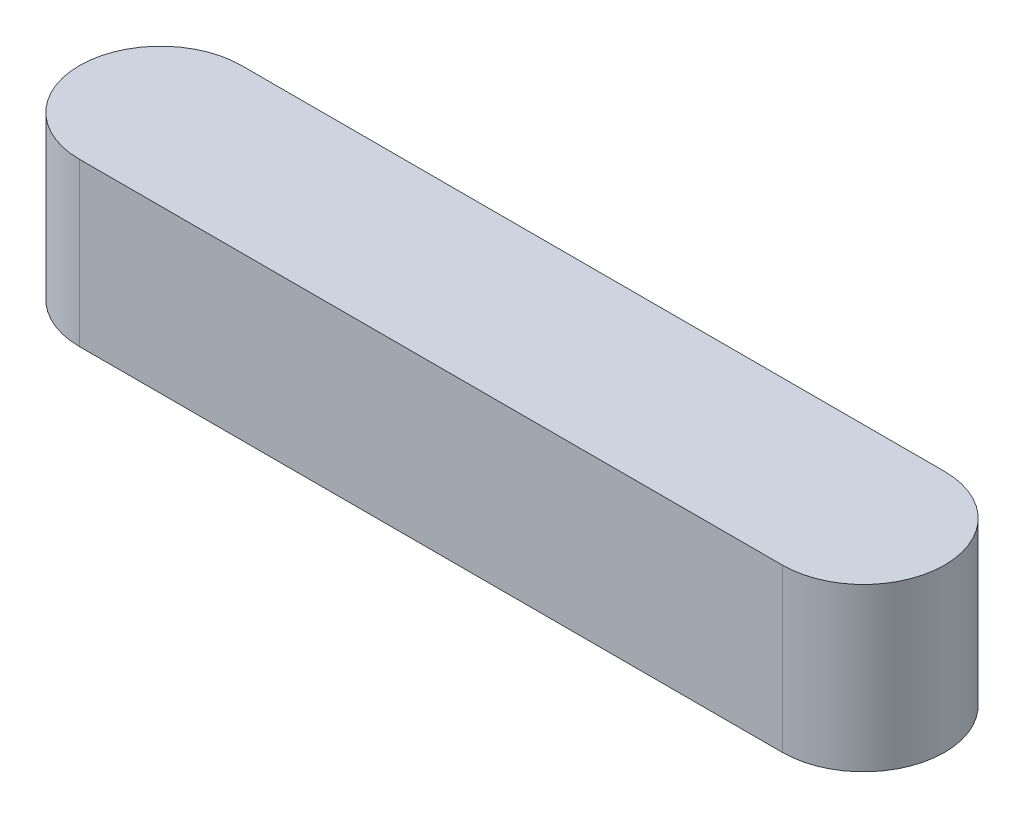
ISO-10303-21;
HEADER;
FILE_DESCRIPTION(('STEP AP214'),'2;1');
FILE_NAME('part.step','',(''),(''),'','','');
FILE_SCHEMA(('AUTOMOTIVE_DESIGN { 1 0 10303 214 1 1 1 1 }'));
ENDSEC;
DATA;
#1=APPLICATION_CONTEXT('core data for automotive mechanical design processes');
#2=APPLICATION_PROTOCOL_DEFINITION('international standard','automotive_design',2000,#1);
#3=PRODUCT_CONTEXT('',#1,'mechanical');
#4=PRODUCT('Part','Part','',(#3));
#5=PRODUCT_RELATED_PRODUCT_CATEGORY('part','',(#4));
#6=PRODUCT_DEFINITION_FORMATION('','',#4);
#7=PRODUCT_DEFINITION_CONTEXT('part definition',#1,'design');
#8=PRODUCT_DEFINITION('design','',#6,#7);
#9=PRODUCT_DEFINITION_SHAPE('','',#8);
#10=(LENGTH_UNIT() NAMED_UNIT(*) SI_UNIT(.MILLI.,.METRE.));
#11=(NAMED_UNIT(*) PLANE_ANGLE_UNIT() SI_UNIT($,.RADIAN.));
#12=(NAMED_UNIT(*) SI_UNIT($,.STERADIAN.) SOLID_ANGLE_UNIT());
#13=UNCERTAINTY_MEASURE_WITH_UNIT(LENGTH_MEASURE(1.E-05),#10,'distance_accuracy_value','');
#14=(GEOMETRIC_REPRESENTATION_CONTEXT(3) GLOBAL_UNCERTAINTY_ASSIGNED_CONTEXT((#13)) GLOBAL_UNIT_ASSIGNED_CONTEXT((#10,
#11,#12)) REPRESENTATION_CONTEXT('',''));
#15=CARTESIAN_POINT('',(0.,0.,0.));
#16=DIRECTION('',(0.,0.,1.));
#17=DIRECTION('',(1.,0.,0.));
#18=AXIS2_PLACEMENT_3D('',#15,#16,#17);
#19=CARTESIAN_POINT('',(-13.,6.,0.));
#20=DIRECTION('',(0.,-1.,0.));
#21=DIRECTION('',(0.,0.,-1.));
#22=AXIS2_PLACEMENT_3D('',#19,#20,#21);
#23=CYLINDRICAL_SURFACE('',#22,3.);
#24=CARTESIAN_POINT('',(-13.,0.,0.));
#25=DIRECTION('',(0.,1.,0.));
#26=DIRECTION('',(0.,0.,1.));
#27=AXIS2_PLACEMENT_3D('',#24,#25,#26);
#28=CIRCLE('',#27,3.);
#29=CARTESIAN_POINT('',(-13.,0.,-3.));
#30=VERTEX_POINT('',#29);
#31=CARTESIAN_POINT('',(-13.,0.,3.));
#32=VERTEX_POINT('',#31);
#33=EDGE_CURVE('E105',#30,#32,#28,.T.);
#34=ORIENTED_EDGE('',*,*,#33,.T.);
#35=DIRECTION('',(0.,-1.,0.));
#36=VECTOR('',#35,1.);
#37=CARTESIAN_POINT('',(-13.,6.,3.));
#38=LINE('',#37,#36);
#39=CARTESIAN_POINT('',(-13.,6.,3.));
#40=VERTEX_POINT('',#39);
#41=EDGE_CURVE('E11',#40,#32,#38,.T.);
#42=ORIENTED_EDGE('',*,*,#41,.F.);
#43=CARTESIAN_POINT('',(-13.,6.,0.));
#44=DIRECTION('',(0.,1.,0.));
#45=DIRECTION('',(0.,0.,1.));
#46=AXIS2_PLACEMENT_3D('',#43,#44,#45);
#47=CIRCLE('',#46,3.);
#48=CARTESIAN_POINT('',(-13.,6.,-3.));
#49=VERTEX_POINT('',#48);
#50=EDGE_CURVE('E89',#49,#40,#47,.T.);
#51=ORIENTED_EDGE('',*,*,#50,.F.);
#52=DIRECTION('',(0.,-1.,0.));
#53=VECTOR('',#52,1.);
#54=CARTESIAN_POINT('',(-13.,6.,-3.));
#55=LINE('',#54,#53);
#56=EDGE_CURVE('E98',#49,#30,#55,.T.);
#57=ORIENTED_EDGE('',*,*,#56,.T.);
#58=EDGE_LOOP('',(#34,#42,#51,#57));
#59=FACE_BOUND('',#58,.T.);
#60=ADVANCED_FACE('F39',(#59),#23,.T.);
#61=CARTESIAN_POINT('',(-13.,6.,3.));
#62=DIRECTION('',(0.,0.,-1.));
#63=DIRECTION('',(-1.,0.,0.));
#64=AXIS2_PLACEMENT_3D('',#61,#62,#63);
#65=PLANE('',#64);
#66=DIRECTION('',(1.,0.,0.));
#67=VECTOR('',#66,1.);
#68=CARTESIAN_POINT('',(-13.,0.,3.));
#69=LINE('',#68,#67);
#70=CARTESIAN_POINT('',(13.,0.,3.));
#71=VERTEX_POINT('',#70);
#72=EDGE_CURVE('E94',#32,#71,#69,.T.);
#73=ORIENTED_EDGE('',*,*,#72,.T.);
#74=DIRECTION('',(0.,-1.,0.));
#75=VECTOR('',#74,1.);
#76=CARTESIAN_POINT('',(13.,6.,3.));
#77=LINE('',#76,#75);
#78=CARTESIAN_POINT('',(13.,6.,3.));
#79=VERTEX_POINT('',#78);
#80=EDGE_CURVE('E50',#79,#71,#77,.T.);
#81=ORIENTED_EDGE('',*,*,#80,.F.);
#82=DIRECTION('',(1.,0.,0.));
#83=VECTOR('',#82,1.);
#84=CARTESIAN_POINT('',(-13.,6.,3.));
#85=LINE('',#84,#83);
#86=EDGE_CURVE('E85',#40,#79,#85,.T.);
#87=ORIENTED_EDGE('',*,*,#86,.F.);
#88=ORIENTED_EDGE('',*,*,#41,.T.);
#89=EDGE_LOOP('',(#73,#81,#87,#88));
#90=FACE_BOUND('',#89,.T.);
#91=ADVANCED_FACE('F91',(#90),#65,.F.);
#92=CARTESIAN_POINT('',(13.,6.,0.));
#93=DIRECTION('',(0.,-1.,0.));
#94=DIRECTION('',(0.,0.,-1.));
#95=AXIS2_PLACEMENT_3D('',#92,#93,#94);
#96=CYLINDRICAL_SURFACE('',#95,3.);
#97=CARTESIAN_POINT('',(13.,0.,0.));
#98=DIRECTION('',(0.,1.,0.));
#99=DIRECTION('',(0.,0.,1.));
#100=AXIS2_PLACEMENT_3D('',#97,#98,#99);
#101=CIRCLE('',#100,3.);
#102=CARTESIAN_POINT('',(13.,0.,-3.));
#103=VERTEX_POINT('',#102);
#104=EDGE_CURVE('E75',#71,#103,#101,.T.);
#105=ORIENTED_EDGE('',*,*,#104,.T.);
#106=DIRECTION('',(0.,-1.,0.));
#107=VECTOR('',#106,1.);
#108=CARTESIAN_POINT('',(13.,6.,-3.));
#109=LINE('',#108,#107);
#110=CARTESIAN_POINT('',(13.,6.,-3.));
#111=VERTEX_POINT('',#110);
#112=EDGE_CURVE('E92',#111,#103,#109,.T.);
#113=ORIENTED_EDGE('',*,*,#112,.F.);
#114=CARTESIAN_POINT('',(13.,6.,0.));
#115=DIRECTION('',(0.,1.,0.));
#116=DIRECTION('',(0.,0.,1.));
#117=AXIS2_PLACEMENT_3D('',#114,#115,#116);
#118=CIRCLE('',#117,3.);
#119=EDGE_CURVE('E86',#79,#111,#118,.T.);
#120=ORIENTED_EDGE('',*,*,#119,.F.);
#121=ORIENTED_EDGE('',*,*,#80,.T.);
#122=EDGE_LOOP('',(#105,#113,#120,#121));
#123=FACE_BOUND('',#122,.T.);
#124=ADVANCED_FACE('F96',(#123),#96,.T.);
#125=CARTESIAN_POINT('',(-13.,6.,-3.));
#126=DIRECTION('',(0.,0.,1.));
#127=DIRECTION('',(1.,0.,0.));
#128=AXIS2_PLACEMENT_3D('',#125,#126,#127);
#129=PLANE('',#128);
#130=DIRECTION('',(-1.,0.,0.));
#131=VECTOR('',#130,1.);
#132=CARTESIAN_POINT('',(-13.,0.,-3.));
#133=LINE('',#132,#131);
#134=EDGE_CURVE('E79',#103,#30,#133,.T.);
#135=ORIENTED_EDGE('',*,*,#134,.T.);
#136=ORIENTED_EDGE('',*,*,#56,.F.);
#137=DIRECTION('',(-1.,0.,0.));
#138=VECTOR('',#137,1.);
#139=CARTESIAN_POINT('',(-13.,6.,-3.));
#140=LINE('',#139,#138);
#141=EDGE_CURVE('E54',#111,#49,#140,.T.);
#142=ORIENTED_EDGE('',*,*,#141,.F.);
#143=ORIENTED_EDGE('',*,*,#112,.T.);
#144=EDGE_LOOP('',(#135,#136,#142,#143));
#145=FACE_BOUND('',#144,.T.);
#146=ADVANCED_FACE('F108',(#145),#129,.F.);
#147=CARTESIAN_POINT('',(-13.,6.,0.));
#148=DIRECTION('',(0.,1.,0.));
#149=DIRECTION('',(0.,0.,1.));
#150=AXIS2_PLACEMENT_3D('',#147,#148,#149);
#151=PLANE('',#150);
#152=ORIENTED_EDGE('',*,*,#50,.T.);
#153=ORIENTED_EDGE('',*,*,#86,.T.);
#154=ORIENTED_EDGE('',*,*,#119,.T.);
#155=ORIENTED_EDGE('',*,*,#141,.T.);
#156=EDGE_LOOP('',(#152,#153,#154,#155));
#157=FACE_BOUND('',#156,.T.);
#158=ADVANCED_FACE('F88',(#157),#151,.T.);
#159=CARTESIAN_POINT('',(-13.,0.,0.));
#160=DIRECTION('',(0.,1.,0.));
#161=DIRECTION('',(0.,0.,1.));
#162=AXIS2_PLACEMENT_3D('',#159,#160,#161);
#163=PLANE('',#162);
#164=ORIENTED_EDGE('',*,*,#33,.F.);
#165=ORIENTED_EDGE('',*,*,#134,.F.);
#166=ORIENTED_EDGE('',*,*,#104,.F.);
#167=ORIENTED_EDGE('',*,*,#72,.F.);
#168=EDGE_LOOP('',(#164,#165,#166,#167));
#169=FACE_BOUND('',#168,.T.);
#170=ADVANCED_FACE('F115',(#169),#163,.F.);
#171=CLOSED_SHELL('',(#60,#91,#124,#146,#158,#170));
#172=MANIFOLD_SOLID_BREP('B2',#171);
#173=ADVANCED_BREP_SHAPE_REPRESENTATION('',(#18,#172),#14);
#174=SHAPE_DEFINITION_REPRESENTATION(#9,#173);
ENDSEC;
END-ISO-10303-21;
